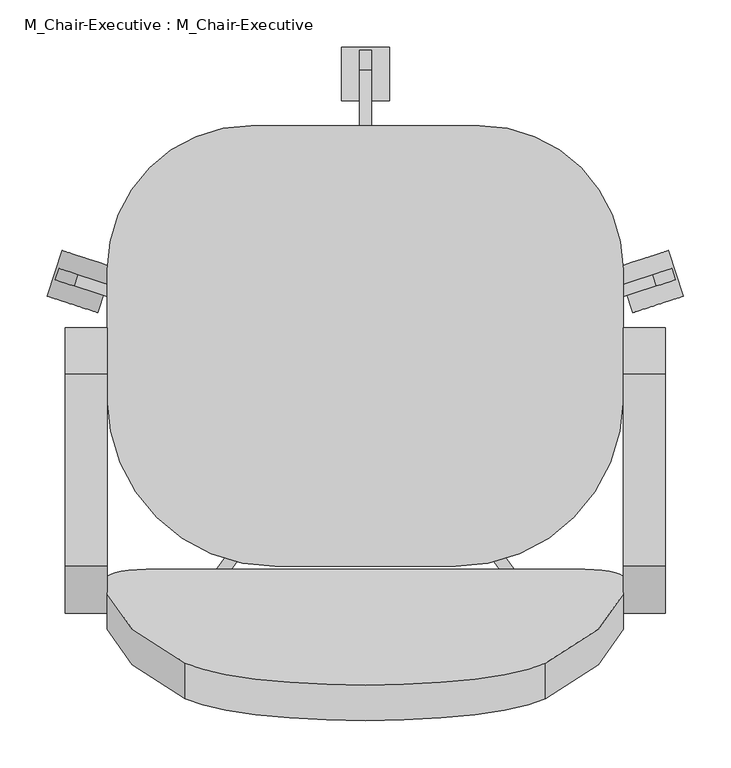
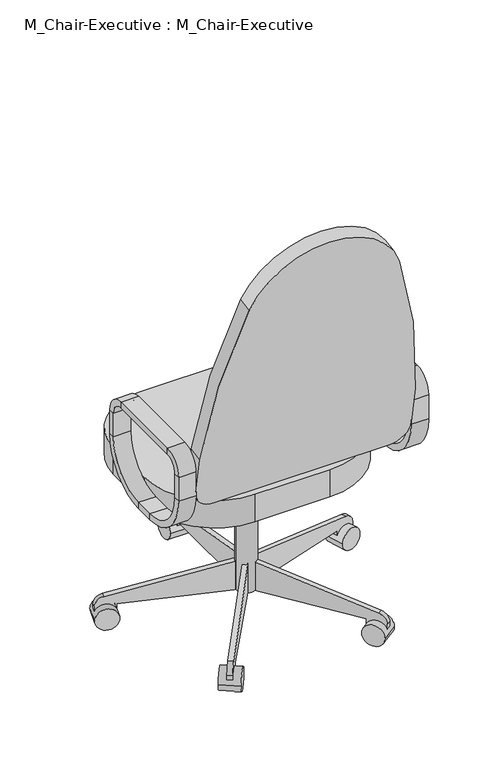
"""IFC4 building model written with IfcOpenShell, lengths in millimetres: furniture geometry, M_Chair-Executive : M_Chair-Executive."""

from ifc_helpers import new_model, si_unit, point, frame, frame_2d, origin, place, context, project, spatial, polyline, circle_curve, trimmed, segment, composite_curve, outline, extrude, source, transform, mapped, element, save
from ifc_brep_helpers import plane_surface, cylinder_surface, revolved_surface, advanced_brep


def m_chair_executive_m_chair_executive_8d69e98c(model_context):
    return source(origin(), model_context, "Body", "SolidModel", [
        advanced_brep(
        [(-176.5091803, -217.7873012, 546.1), (-176.5091803, -108.0540984, 436.3667972), (-176.5091803, -108.0540984, 420.4917972), (-176.5091803, -233.6623012, 546.1), (-132.0591803, -217.7873012, 546.1), (-132.0591803, -108.0540984, 436.3667972), (-132.0591803, -233.6623012, 546.1), (-132.0591803, -108.0540984, 420.4917972), (-176.5091803, -233.6623012, 609.6), (-176.5091803, -217.7873012, 609.6), (-132.0591803, -217.7873012, 609.6), (-132.0591803, -233.6623012, 609.6), (-176.5091803, -184.2540984, 643.1332028), (-176.5091803, -184.2540984, 659.0082028), (-132.0591803, -184.2540984, 643.1332028), (-132.0591803, -184.2540984, 659.0082028), (-176.5091803, 18.9459016, 659.0082028), (-176.5091803, 18.9459016, 643.1332028), (-132.0591803, 18.9459016, 643.1332028), (-132.0591803, 18.9459016, 659.0082028), (-176.5091803, 52.4791044, 609.6), (-176.5091803, 68.3541044, 609.6), (-132.0591803, 52.4791044, 609.6), (-132.0591803, 68.3541044, 609.6), (-176.5091803, 68.3541044, 546.1), (-176.5091803, 52.4791044, 546.1), (-132.0591803, 52.4791044, 546.1), (-132.0591803, 68.3541044, 546.1), (-176.5091803, -57.2540984, 436.3667972), (-176.5091803, -57.2540984, 420.4917972), (-132.0591803, -57.2540984, 436.3667972), (-132.0591803, -57.2540984, 420.4917972)],
        [
            (0, 1, circle_curve(frame((-176.5091803, -108.0540984, 546.1), z_axis=(1.0, 0.0, 0.0), x_axis=(0.0, 0.0, -1.0)), 109.7332028)),
            (1, 2),
            (2, 3, circle_curve(frame((-176.5091803, -108.0540984, 546.1), z_axis=(-1.0, 0.0, 0.0), x_axis=(0.0, 0.0, -1.0)), 125.6082028)),
            (3, 0),
            (4, 5, circle_curve(frame((-132.0591803, -108.0540984, 546.1), z_axis=(1.0, 0.0, 0.0), x_axis=(0.0, 0.0, -1.0)), 109.7332028)),
            (5, 1),
            (0, 4),
            (6, 7, circle_curve(frame((-132.0591803, -108.0540984, 546.1), z_axis=(1.0, 0.0, 0.0), x_axis=(0.0, 0.0, -1.0)), 125.6082028)),
            (7, 5),
            (4, 6),
            (2, 7),
            (6, 3),
            (3, 8),
            (8, 9),
            (9, 0),
            (9, 10),
            (10, 4),
            (10, 11),
            (11, 6),
            (11, 8),
            (12, 9, circle_curve(frame((-176.5091803, -184.2540984, 609.6), z_axis=(1.0, 0.0, 0.0), x_axis=(0.0, -1.0, 0.0)), 33.5332028)),
            (8, 13, circle_curve(frame((-176.5091803, -184.2540984, 609.6), z_axis=(-1.0, 0.0, 0.0), x_axis=(0.0, -1.0, 0.0)), 49.4082028)),
            (13, 12),
            (14, 10, circle_curve(frame((-132.0591803, -184.2540984, 609.6), z_axis=(1.0, 0.0, 0.0), x_axis=(0.0, -1.0, 0.0)), 33.5332028)),
            (12, 14),
            (15, 11, circle_curve(frame((-132.0591803, -184.2540984, 609.6), z_axis=(1.0, 0.0, 0.0), x_axis=(0.0, -1.0, 0.0)), 49.4082028)),
            (14, 15),
            (15, 13),
            (13, 16),
            (16, 17),
            (17, 12),
            (17, 18),
            (18, 14),
            (18, 19),
            (19, 15),
            (19, 16),
            (20, 17, circle_curve(frame((-176.5091803, 18.9459016, 609.6), z_axis=(1.0, 0.0, 0.0), x_axis=(0.0, 0.0, 1.0)), 33.5332028)),
            (16, 21, circle_curve(frame((-176.5091803, 18.9459016, 609.6), z_axis=(-1.0, 0.0, 0.0), x_axis=(0.0, 0.0, 1.0)), 49.4082028)),
            (21, 20),
            (22, 18, circle_curve(frame((-132.0591803, 18.9459016, 609.6), z_axis=(1.0, 0.0, 0.0), x_axis=(0.0, 0.0, 1.0)), 33.5332028)),
            (20, 22),
            (23, 19, circle_curve(frame((-132.0591803, 18.9459016, 609.6), z_axis=(1.0, 0.0, 0.0), x_axis=(0.0, 0.0, 1.0)), 49.4082028)),
            (22, 23),
            (23, 21),
            (21, 24),
            (24, 25),
            (25, 20),
            (25, 26),
            (26, 22),
            (26, 27),
            (27, 23),
            (27, 24),
            (28, 25, circle_curve(frame((-176.5091803, -57.2540984, 546.1), z_axis=(1.0, 0.0, 0.0), x_axis=(0.0, 1.0, 0.0)), 109.7332028)),
            (24, 29, circle_curve(frame((-176.5091803, -57.2540984, 546.1), z_axis=(-1.0, 0.0, 0.0), x_axis=(0.0, 1.0, 0.0)), 125.6082028)),
            (29, 28),
            (30, 26, circle_curve(frame((-132.0591803, -57.2540984, 546.1), z_axis=(1.0, 0.0, 0.0), x_axis=(0.0, 1.0, 0.0)), 109.7332028)),
            (28, 30),
            (31, 27, circle_curve(frame((-132.0591803, -57.2540984, 546.1), z_axis=(1.0, 0.0, 0.0), x_axis=(0.0, 1.0, 0.0)), 125.6082028)),
            (30, 31),
            (31, 29),
            (29, 2),
            (1, 28),
            (5, 30),
            (7, 31),
        ],
        [
            plane_surface(frame((-176.5091803, -108.0540984, 546.1), z_axis=(-1.0, 0.0, 0.0), x_axis=(0.0, 0.0, -1.0))),
            revolved_surface(polyline([(-176.5091803, -108.0540984, 436.3667972), (-132.0591803, -108.0540984, 436.3667972)]), (-132.0591803, -108.0540984, 546.1), (-1.0, 0.0, 0.0)),
            plane_surface(frame((-132.0591803, -108.0540984, 546.1), z_axis=(1.0, 0.0, 0.0), x_axis=(0.0, 0.0, -1.0))),
            cylinder_surface(frame((-132.0591803, -108.0540984, 546.1), z_axis=(-1.0, 0.0, 0.0), x_axis=(0.0, 0.0, -1.0)), 125.6082028),
            plane_surface(frame((-176.5091803, -233.6623012, 546.1), z_axis=(-1.0, 0.0, 0.0), x_axis=(0.0, 0.0, 1.0))),
            plane_surface(frame((-176.5091803, -217.7873012, 546.1), z_axis=(0.0, 1.0, 0.0), x_axis=(0.0, 0.0, 1.0))),
            plane_surface(frame((-132.0591803, -217.7873012, 546.1), z_axis=(1.0, 0.0, 0.0), x_axis=(0.0, 0.0, 1.0))),
            plane_surface(frame((-132.0591803, -233.6623012, 546.1), z_axis=(0.0, -1.0, 0.0), x_axis=(0.0, 0.0, 1.0))),
            plane_surface(frame((-176.5091803, -184.2540984, 609.6), z_axis=(-1.0, 0.0, 0.0), x_axis=(0.0, -1.0, 0.0))),
            revolved_surface(polyline([(-176.5091803, -217.7873012, 609.6), (-132.0591803, -217.7873012, 609.6)]), (-132.0591803, -184.2540984, 609.6), (-1.0, 0.0, 0.0)),
            plane_surface(frame((-132.0591803, -184.2540984, 609.6), z_axis=(1.0, 0.0, 0.0), x_axis=(0.0, -1.0, 0.0))),
            cylinder_surface(frame((-132.0591803, -184.2540984, 609.6), z_axis=(-1.0, 0.0, 0.0), x_axis=(0.0, -1.0, 0.0)), 49.4082028),
            plane_surface(frame((-176.5091803, -184.2540984, 659.0082028), z_axis=(-1.0, 0.0, 0.0), x_axis=(0.0, 1.0, 0.0))),
            plane_surface(frame((-176.5091803, -184.2540984, 643.1332028), z_axis=(0.0, 0.0, -1.0), x_axis=(0.0, 1.0, 0.0))),
            plane_surface(frame((-132.0591803, -184.2540984, 643.1332028), z_axis=(1.0, 0.0, 0.0), x_axis=(0.0, 1.0, 0.0))),
            plane_surface(frame((-132.0591803, -184.2540984, 659.0082028), z_axis=(0.0, 0.0, 1.0), x_axis=(0.0, 1.0, 0.0))),
            plane_surface(frame((-176.5091803, 18.9459016, 609.6), z_axis=(-1.0, 0.0, 0.0), x_axis=(0.0, 0.0, 1.0))),
            revolved_surface(polyline([(-176.5091803, 18.9459016, 643.1332028), (-132.0591803, 18.9459016, 643.1332028)]), (-132.0591803, 18.9459016, 609.6), (-1.0, 0.0, 0.0)),
            plane_surface(frame((-132.0591803, 18.9459016, 609.6), z_axis=(1.0, 0.0, 0.0), x_axis=(0.0, 0.0, 1.0))),
            cylinder_surface(frame((-132.0591803, 18.9459016, 609.6), z_axis=(-1.0, 0.0, 0.0), x_axis=(0.0, 0.0, 1.0)), 49.4082028),
            plane_surface(frame((-176.5091803, 68.3541044, 609.6), z_axis=(-1.0, 0.0, 0.0), x_axis=(0.0, 0.0, -1.0))),
            plane_surface(frame((-176.5091803, 52.4791044, 609.6), z_axis=(0.0, -1.0, 0.0), x_axis=(0.0, 0.0, -1.0))),
            plane_surface(frame((-132.0591803, 52.4791044, 609.6), z_axis=(1.0, 0.0, 0.0), x_axis=(0.0, 0.0, -1.0))),
            plane_surface(frame((-132.0591803, 68.3541044, 609.6), z_axis=(0.0, 1.0, 0.0), x_axis=(0.0, 0.0, -1.0))),
            plane_surface(frame((-176.5091803, -57.2540984, 546.1), z_axis=(-1.0, 0.0, 0.0), x_axis=(0.0, 1.0, 0.0))),
            revolved_surface(polyline([(-176.5091803, 52.479104400000004, 546.1), (-132.0591803, 52.479104400000004, 546.1)]), (-132.0591803, -57.2540984, 546.1), (-1.0, 0.0, 0.0)),
            plane_surface(frame((-132.0591803, -57.2540984, 546.1), z_axis=(1.0, 0.0, 0.0), x_axis=(0.0, 1.0, 0.0))),
            cylinder_surface(frame((-132.0591803, -57.2540984, 546.1), z_axis=(-1.0, 0.0, 0.0), x_axis=(0.0, 1.0, 0.0)), 125.6082028),
            plane_surface(frame((-176.5091803, -57.2540984, 420.4917972), z_axis=(-1.0, 0.0, 0.0), x_axis=(0.0, -1.0, 0.0))),
            plane_surface(frame((-176.5091803, -57.2540984, 436.3667972), z_axis=(0.0, 0.0, 1.0), x_axis=(0.0, -1.0, 0.0))),
            plane_surface(frame((-132.0591803, -57.2540984, 436.3667972), z_axis=(1.0, 0.0, 0.0), x_axis=(0.0, -1.0, 0.0))),
            plane_surface(frame((-132.0591803, -57.2540984, 420.4917972), z_axis=(0.0, 0.0, -1.0), x_axis=(0.0, -1.0, 0.0))),
        ],
        [
            (0, [[1, 2, 3, 4]]),
            (1, [[5, 6, -1, 7]]),
            (2, [[8, 9, -5, 10]]),
            (3, [[-3, 11, -8, 12]]),
            (4, [[-4, 13, 14, 15]]),
            (5, [[-7, -15, 16, 17]]),
            (6, [[-10, -17, 18, 19]]),
            (7, [[-12, -19, 20, -13]]),
            (8, [[21, -14, 22, 23]]),
            (9, [[24, -16, -21, 25]]),
            (10, [[26, -18, -24, 27]]),
            (11, [[-22, -20, -26, 28]]),
            (12, [[-23, 29, 30, 31]]),
            (13, [[-25, -31, 32, 33]]),
            (14, [[-27, -33, 34, 35]]),
            (15, [[-28, -35, 36, -29]]),
            (16, [[37, -30, 38, 39]]),
            (17, [[40, -32, -37, 41]]),
            (18, [[42, -34, -40, 43]]),
            (19, [[-38, -36, -42, 44]]),
            (20, [[-39, 45, 46, 47]]),
            (21, [[-41, -47, 48, 49]]),
            (22, [[-43, -49, 50, 51]]),
            (23, [[-44, -51, 52, -45]]),
            (24, [[53, -46, 54, 55]]),
            (25, [[56, -48, -53, 57]]),
            (26, [[58, -50, -56, 59]]),
            (27, [[-54, -52, -58, 60]]),
            (28, [[-55, 61, -2, 62]]),
            (29, [[-57, -62, -6, 63]]),
            (30, [[-59, -63, -9, 64]]),
            (31, [[-60, -64, -11, -61]]),
        ],
    ),
        advanced_brep(
        [(414.0408197, -233.6623012, 546.1), (414.0408197, -108.0540984, 420.4917972), (458.4908197, -108.0540984, 420.4917972), (458.4908197, -233.6623012, 546.1), (414.0408197, -217.7873012, 546.1), (414.0408197, -108.0540984, 436.3667972), (458.4908197, -217.7873012, 546.1), (458.4908197, -108.0540984, 436.3667972), (458.4908197, -233.6623012, 609.6), (414.0408197, -233.6623012, 609.6), (414.0408197, -217.7873012, 609.6), (458.4908197, -217.7873012, 609.6), (414.0408197, -184.2540984, 659.0082028), (458.4908197, -184.2540984, 659.0082028), (414.0408197, -184.2540984, 643.1332028), (458.4908197, -184.2540984, 643.1332028), (458.4908197, 18.9459016, 659.0082028), (414.0408197, 18.9459016, 659.0082028), (414.0408197, 18.9459016, 643.1332028), (458.4908197, 18.9459016, 643.1332028), (414.0408197, 68.3541044, 609.6), (458.4908197, 68.3541044, 609.6), (414.0408197, 52.4791044, 609.6), (458.4908197, 52.4791044, 609.6), (458.4908197, 68.3541044, 546.1), (414.0408197, 68.3541044, 546.1), (414.0408197, 52.4791044, 546.1), (458.4908197, 52.4791044, 546.1), (414.0408197, -57.2540984, 420.4917972), (458.4908197, -57.2540984, 420.4917972), (414.0408197, -57.2540984, 436.3667972), (458.4908197, -57.2540984, 436.3667972)],
        [
            (0, 1, circle_curve(frame((414.0408197, -108.0540984, 546.1), z_axis=(1.0, 0.0, 0.0), x_axis=(0.0, 0.0, -1.0)), 125.6082028)),
            (1, 2),
            (2, 3, circle_curve(frame((458.4908197, -108.0540984, 546.1), z_axis=(-1.0, 0.0, 0.0), x_axis=(0.0, 0.0, -1.0)), 125.6082028)),
            (3, 0),
            (4, 5, circle_curve(frame((414.0408197, -108.0540984, 546.1), z_axis=(1.0, 0.0, 0.0), x_axis=(0.0, 0.0, -1.0)), 109.7332028)),
            (5, 1),
            (0, 4),
            (6, 7, circle_curve(frame((458.4908197, -108.0540984, 546.1), z_axis=(1.0, 0.0, 0.0), x_axis=(0.0, 0.0, -1.0)), 109.7332028)),
            (7, 5),
            (4, 6),
            (2, 7),
            (6, 3),
            (3, 8),
            (8, 9),
            (9, 0),
            (9, 10),
            (10, 4),
            (10, 11),
            (11, 6),
            (11, 8),
            (12, 9, circle_curve(frame((414.0408197, -184.2540984, 609.6), z_axis=(1.0, 0.0, 0.0), x_axis=(0.0, -1.0, 0.0)), 49.4082028)),
            (8, 13, circle_curve(frame((458.4908197, -184.2540984, 609.6), z_axis=(-1.0, 0.0, 0.0), x_axis=(0.0, -1.0, 0.0)), 49.4082028)),
            (13, 12),
            (14, 10, circle_curve(frame((414.0408197, -184.2540984, 609.6), z_axis=(1.0, 0.0, 0.0), x_axis=(0.0, -1.0, 0.0)), 33.5332028)),
            (12, 14),
            (15, 11, circle_curve(frame((458.4908197, -184.2540984, 609.6), z_axis=(1.0, 0.0, 0.0), x_axis=(0.0, -1.0, 0.0)), 33.5332028)),
            (14, 15),
            (15, 13),
            (13, 16),
            (16, 17),
            (17, 12),
            (17, 18),
            (18, 14),
            (18, 19),
            (19, 15),
            (19, 16),
            (20, 17, circle_curve(frame((414.0408197, 18.9459016, 609.6), z_axis=(1.0, 0.0, 0.0), x_axis=(0.0, 0.0, 1.0)), 49.4082028)),
            (16, 21, circle_curve(frame((458.4908197, 18.9459016, 609.6), z_axis=(-1.0, 0.0, 0.0), x_axis=(0.0, 0.0, 1.0)), 49.4082028)),
            (21, 20),
            (22, 18, circle_curve(frame((414.0408197, 18.9459016, 609.6), z_axis=(1.0, 0.0, 0.0), x_axis=(0.0, 0.0, 1.0)), 33.5332028)),
            (20, 22),
            (23, 19, circle_curve(frame((458.4908197, 18.9459016, 609.6), z_axis=(1.0, 0.0, 0.0), x_axis=(0.0, 0.0, 1.0)), 33.5332028)),
            (22, 23),
            (23, 21),
            (21, 24),
            (24, 25),
            (25, 20),
            (25, 26),
            (26, 22),
            (26, 27),
            (27, 23),
            (27, 24),
            (28, 25, circle_curve(frame((414.0408197, -57.2540984, 546.1), z_axis=(1.0, 0.0, 0.0), x_axis=(0.0, 1.0, 0.0)), 125.6082028)),
            (24, 29, circle_curve(frame((458.4908197, -57.2540984, 546.1), z_axis=(-1.0, 0.0, 0.0), x_axis=(0.0, 1.0, 0.0)), 125.6082028)),
            (29, 28),
            (30, 26, circle_curve(frame((414.0408197, -57.2540984, 546.1), z_axis=(1.0, 0.0, 0.0), x_axis=(0.0, 1.0, 0.0)), 109.7332028)),
            (28, 30),
            (31, 27, circle_curve(frame((458.4908197, -57.2540984, 546.1), z_axis=(1.0, 0.0, 0.0), x_axis=(0.0, 1.0, 0.0)), 109.7332028)),
            (30, 31),
            (31, 29),
            (29, 2),
            (1, 28),
            (5, 30),
            (7, 31),
        ],
        [
            cylinder_surface(frame((414.0408197, -108.0540984, 546.1), z_axis=(-1.0, 0.0, 0.0), x_axis=(0.0, 0.0, -1.0)), 125.6082028),
            plane_surface(frame((414.0408197, -108.0540984, 546.1), z_axis=(-1.0, 0.0, 0.0), x_axis=(0.0, 0.0, -1.0))),
            revolved_surface(polyline([(414.0408197, -108.0540984, 436.3667972), (458.4908197, -108.0540984, 436.3667972)]), (414.0408197, -108.0540984, 546.1), (-1.0, 0.0, 0.0)),
            plane_surface(frame((458.4908197, -108.0540984, 546.1), z_axis=(1.0, 0.0, 0.0), x_axis=(0.0, 0.0, -1.0))),
            plane_surface(frame((458.4908197, -233.6623012, 546.1), z_axis=(0.0, -1.0, 0.0), x_axis=(0.0, 0.0, 1.0))),
            plane_surface(frame((414.0408197, -233.6623012, 546.1), z_axis=(-1.0, 0.0, 0.0), x_axis=(0.0, 0.0, 1.0))),
            plane_surface(frame((414.0408197, -217.7873012, 546.1), z_axis=(0.0, 1.0, 0.0), x_axis=(0.0, 0.0, 1.0))),
            plane_surface(frame((458.4908197, -217.7873012, 546.1), z_axis=(1.0, 0.0, 0.0), x_axis=(0.0, 0.0, 1.0))),
            cylinder_surface(frame((414.0408197, -184.2540984, 609.6), z_axis=(-1.0, 0.0, 0.0), x_axis=(0.0, -1.0, 0.0)), 49.4082028),
            plane_surface(frame((414.0408197, -184.2540984, 609.6), z_axis=(-1.0, 0.0, 0.0), x_axis=(0.0, -1.0, 0.0))),
            revolved_surface(polyline([(414.0408197, -217.7873012, 609.6), (458.4908197, -217.7873012, 609.6)]), (414.0408197, -184.2540984, 609.6), (-1.0, 0.0, 0.0)),
            plane_surface(frame((458.4908197, -184.2540984, 609.6), z_axis=(1.0, 0.0, 0.0), x_axis=(0.0, -1.0, 0.0))),
            plane_surface(frame((458.4908197, -184.2540984, 659.0082028), z_axis=(0.0, 0.0, 1.0), x_axis=(0.0, 1.0, 0.0))),
            plane_surface(frame((414.0408197, -184.2540984, 659.0082028), z_axis=(-1.0, 0.0, 0.0), x_axis=(0.0, 1.0, 0.0))),
            plane_surface(frame((414.0408197, -184.2540984, 643.1332028), z_axis=(0.0, 0.0, -1.0), x_axis=(0.0, 1.0, 0.0))),
            plane_surface(frame((458.4908197, -184.2540984, 643.1332028), z_axis=(1.0, 0.0, 0.0), x_axis=(0.0, 1.0, 0.0))),
            cylinder_surface(frame((414.0408197, 18.9459016, 609.6), z_axis=(-1.0, 0.0, 0.0), x_axis=(0.0, 0.0, 1.0)), 49.4082028),
            plane_surface(frame((414.0408197, 18.9459016, 609.6), z_axis=(-1.0, 0.0, 0.0), x_axis=(0.0, 0.0, 1.0))),
            revolved_surface(polyline([(414.0408197, 18.9459016, 643.1332028), (458.4908197, 18.9459016, 643.1332028)]), (414.0408197, 18.9459016, 609.6), (-1.0, 0.0, 0.0)),
            plane_surface(frame((458.4908197, 18.9459016, 609.6), z_axis=(1.0, 0.0, 0.0), x_axis=(0.0, 0.0, 1.0))),
            plane_surface(frame((458.4908197, 68.3541044, 609.6), z_axis=(0.0, 1.0, 0.0), x_axis=(0.0, 0.0, -1.0))),
            plane_surface(frame((414.0408197, 68.3541044, 609.6), z_axis=(-1.0, 0.0, 0.0), x_axis=(0.0, 0.0, -1.0))),
            plane_surface(frame((414.0408197, 52.4791044, 609.6), z_axis=(0.0, -1.0, 0.0), x_axis=(0.0, 0.0, -1.0))),
            plane_surface(frame((458.4908197, 52.4791044, 609.6), z_axis=(1.0, 0.0, 0.0), x_axis=(0.0, 0.0, -1.0))),
            cylinder_surface(frame((414.0408197, -57.2540984, 546.1), z_axis=(-1.0, 0.0, 0.0), x_axis=(0.0, 1.0, 0.0)), 125.6082028),
            plane_surface(frame((414.0408197, -57.2540984, 546.1), z_axis=(-1.0, 0.0, 0.0), x_axis=(0.0, 1.0, 0.0))),
            revolved_surface(polyline([(414.0408197, 52.479104400000004, 546.1), (458.4908197, 52.479104400000004, 546.1)]), (414.0408197, -57.2540984, 546.1), (-1.0, 0.0, 0.0)),
            plane_surface(frame((458.4908197, -57.2540984, 546.1), z_axis=(1.0, 0.0, 0.0), x_axis=(0.0, 1.0, 0.0))),
            plane_surface(frame((458.4908197, -57.2540984, 420.4917972), z_axis=(0.0, 0.0, -1.0), x_axis=(0.0, -1.0, 0.0))),
            plane_surface(frame((414.0408197, -57.2540984, 420.4917972), z_axis=(-1.0, 0.0, 0.0), x_axis=(0.0, -1.0, 0.0))),
            plane_surface(frame((414.0408197, -57.2540984, 436.3667972), z_axis=(0.0, 0.0, 1.0), x_axis=(0.0, -1.0, 0.0))),
            plane_surface(frame((458.4908197, -57.2540984, 436.3667972), z_axis=(1.0, 0.0, 0.0), x_axis=(0.0, -1.0, 0.0))),
        ],
        [
            (0, [[1, 2, 3, 4]]),
            (1, [[5, 6, -1, 7]]),
            (2, [[8, 9, -5, 10]]),
            (3, [[-3, 11, -8, 12]]),
            (4, [[-4, 13, 14, 15]]),
            (5, [[-7, -15, 16, 17]]),
            (6, [[-10, -17, 18, 19]]),
            (7, [[-12, -19, 20, -13]]),
            (8, [[21, -14, 22, 23]]),
            (9, [[24, -16, -21, 25]]),
            (10, [[26, -18, -24, 27]]),
            (11, [[-22, -20, -26, 28]]),
            (12, [[-23, 29, 30, 31]]),
            (13, [[-25, -31, 32, 33]]),
            (14, [[-27, -33, 34, 35]]),
            (15, [[-28, -35, 36, -29]]),
            (16, [[37, -30, 38, 39]]),
            (17, [[40, -32, -37, 41]]),
            (18, [[42, -34, -40, 43]]),
            (19, [[-38, -36, -42, 44]]),
            (20, [[-39, 45, 46, 47]]),
            (21, [[-41, -47, 48, 49]]),
            (22, [[-43, -49, 50, 51]]),
            (23, [[-44, -51, 52, -45]]),
            (24, [[53, -46, 54, 55]]),
            (25, [[56, -48, -53, 57]]),
            (26, [[58, -50, -56, 59]]),
            (27, [[-54, -52, -58, 60]]),
            (28, [[-55, 61, -2, 62]]),
            (29, [[-57, -62, -6, 63]]),
            (30, [[-59, -63, -9, 64]]),
            (31, [[-60, -64, -11, -61]]),
        ],
    ),
        extrude(outline(composite_curve([segment(trimmed(circle_curve(frame_2d((0.0, -50.8)), 50.8), [point((0.0, 0.0))], [point((50.8, -50.8))], False, "CARTESIAN"), True, "CONTINUOUS"), segment(polyline([(50.8, -50.8), (50.8, -152.4)]), True, "CONTINUOUS"), segment(trimmed(circle_curve(frame_2d((-1471.2021854, -74.3913617)), 1524.0), [point((50.8, -152.4))], [point((-31.75, -574.9444618))], False, "CARTESIAN"), True, "CONTINUOUS"), segment(trimmed(circle_curve(frame_2d((-222.25, -504.2338544)), 203.2), [point((-31.75, -574.9444618))], [point((-412.75, -574.9444618))], False, "CARTESIAN"), True, "CONTINUOUS"), segment(trimmed(circle_curve(frame_2d((1026.7021854, -74.3913617)), 1524.0), [point((-412.75, -574.9444618))], [point((-495.3, -152.4))], False, "CARTESIAN"), True, "CONTINUOUS"), segment(polyline([(-495.3, -152.4), (-495.3, -50.8)]), True, "CONTINUOUS"), segment(trimmed(circle_curve(frame_2d((-444.5, -50.8)), 50.8), [point((-495.3, -50.8))], [point((-444.5, 0.0))], False, "CARTESIAN"), True, "CONTINUOUS"), segment(polyline([(-444.5, 0.0), (0.0, 0.0)]), True, "CONTINUOUS")], self_intersect=False)), frame((363.2408197, -224.5698964, 503.1641822), z_axis=(0.0, 0.9848077530122084, 0.17364817766692853), x_axis=(1.0, 0.0, 0.0)), (0.0, 0.0, 1.0), 38.1),
        extrude(outline(composite_curve([segment(trimmed(circle_curve(frame_2d((20.3408197, 129.4961016)), 152.4), [point((-132.0591803, 129.4961016))], [point((20.3408197, 281.8961016))], False, "CARTESIAN"), True, "CONTINUOUS"), segment(polyline([(20.3408197, 281.8961016), (261.6408197, 281.8961016)]), True, "CONTINUOUS"), segment(trimmed(circle_curve(frame_2d((261.6408197, 129.4961016)), 152.4), [point((261.6408197, 281.8961016))], [point((414.0408197, 129.4961016))], False, "CARTESIAN"), True, "CONTINUOUS"), segment(polyline([(414.0408197, 129.4961016), (414.0408197, -6.4540984)]), True, "CONTINUOUS"), segment(trimmed(circle_curve(frame_2d((236.2408197, -6.4540984)), 177.8), [point((414.0408197, -6.4540984))], [point((236.2408197, -184.2540984))], False, "CARTESIAN"), True, "CONTINUOUS"), segment(polyline([(236.2408197, -184.2540984), (45.7408197, -184.2540984)]), True, "CONTINUOUS"), segment(trimmed(circle_curve(frame_2d((45.7408197, -6.4540984)), 177.8), [point((45.7408197, -184.2540984))], [point((-132.0591803, -6.4540984))], False, "CARTESIAN"), True, "CONTINUOUS"), segment(polyline([(-132.0591803, -6.4540984), (-132.0591803, 129.4961016)]), True, "CONTINUOUS")], self_intersect=False)), frame((0.0, 0.0, 383.7835944), z_axis=(0.0, 0.0, 1.0), x_axis=(1.0, 0.0, 0.0)), (0.0, 0.0, 1.0), 73.4164056),
        extrude(outline(composite_curve([segment(trimmed(circle_curve(frame_2d((140.9908197, 18.9459016)), 25.4), [point((115.5908197, 18.9459016))], [point((166.3908197, 18.9459016))], False, "CARTESIAN"), True, "CONTINUOUS"), segment(trimmed(circle_curve(frame_2d((140.9908197, 18.9459016)), 25.4), [point((166.3908197, 18.9459016))], [point((115.5908197, 18.9459016))], False, "CARTESIAN"), True, "CONTINUOUS")], self_intersect=False)), frame((0.0, 0.0, 53.5835944), z_axis=(0.0, 0.0, 1.0), x_axis=(1.0, 0.0, 0.0)), (0.0, 0.0, 1.0), 330.5914056),
        extrude(outline(composite_curve([segment(trimmed(circle_curve(frame_2d((0.0, -28.2002727)), 28.2002727), [point((0.0, -56.4005455))], [point((0.0, 0.0))], False, "CARTESIAN"), True, "CONTINUOUS"), segment(trimmed(circle_curve(frame_2d((0.0, -28.2002727)), 28.2002727), [point((0.0, 0.0))], [point((0.0, -56.4005455))], False, "CARTESIAN"), True, "CONTINUOUS")], self_intersect=False)), frame((477.6203484, 101.6163254, 28.1835944), z_axis=(-0.3090169943749423, 0.9510565162951553, 0.0), x_axis=(0.0, 0.0, 1.0)), (0.0, 0.0, 1.0), 50.8),
        extrude(outline(composite_curve([segment(polyline([(-25.4, 0.0), (0.0, 0.0), (0.0, -50.8), (-24.303053, -50.8)]), True, "CONTINUOUS"), segment(trimmed(circle_curve(frame_2d((-24.303053, -25.4)), 25.4), [point((-24.303053, -50.8))], [point((-49.3171699, -29.8106637))], False, "CARTESIAN"), True, "CONTINUOUS"), segment(polyline([(-49.3171699, -29.8106637), (-101.6, 266.7), (-101.6, 292.1), (-25.4, 292.1), (-25.4, 0.0)]), True, "CONTINUOUS")], self_intersect=False)), frame((420.756686, 103.1705568, 28.1835944), z_axis=(-0.3090169943749423, 0.9510565162951553, 0.0), x_axis=(0.0, 0.0, -1.0)), (0.0, 0.0, 1.0), 12.7),
        extrude(outline(composite_curve([segment(trimmed(circle_curve(frame_2d((0.0, -28.2002727)), 28.2002727), [point((0.0, -56.4005455))], [point((0.0, 0.0))], False, "CARTESIAN"), True, "CONTINUOUS"), segment(trimmed(circle_curve(frame_2d((0.0, -28.2002727)), 28.2002727), [point((0.0, 0.0))], [point((0.0, -56.4005455))], False, "CARTESIAN"), True, "CONTINUOUS")], self_intersect=False)), frame((323.63931, -275.6612394, 28.1835944), z_axis=(0.8090169943749499, 0.5877852522924699, 0.0), x_axis=(0.0, 0.0, 1.0)), (0.0, 0.0, 1.0), 50.8),
        extrude(outline(composite_curve([segment(polyline([(-25.4, 0.0), (0.0, 0.0), (0.0, -50.8), (-24.303053, -50.8)]), True, "CONTINUOUS"), segment(trimmed(circle_curve(frame_2d((-24.303053, -25.3999999)), 25.4), [point((-24.303053, -50.8))], [point((-49.3171699, -29.8106636))], False, "CARTESIAN"), True, "CONTINUOUS"), segment(polyline([(-49.3171699, -29.8106636), (-101.6, 266.7), (-101.6, 292.1), (-25.4, 292.1), (-25.4, 0.0)]), True, "CONTINUOUS")], self_intersect=False)), frame((307.545634, -221.1003988, 28.1835944), z_axis=(0.8090169943749499, 0.5877852522924699, 0.0), x_axis=(0.0, 0.0, -1.0)), (0.0, 0.0, 1.0), 12.7),
        extrude(outline(composite_curve([segment(trimmed(circle_curve(frame_2d((0.0, -28.2002727)), 28.2002727), [point((0.0, -56.4005455))], [point((0.0, 0.0))], False, "CARTESIAN"), True, "CONTINUOUS"), segment(trimmed(circle_curve(frame_2d((0.0, -28.2002727)), 28.2002727), [point((0.0, 0.0))], [point((0.0, -56.4005455))], False, "CARTESIAN"), True, "CONTINUOUS")], self_intersect=False)), frame((-41.6576707, -275.6612394, 28.1835944), z_axis=(-0.8090169943749458, 0.5877852522924754, 0.0), x_axis=(0.0, 0.0, -1.0)), (0.0, 0.0, 1.0), 50.8),
        extrude(outline(composite_curve([segment(polyline([(25.4, 0.0), (25.4, 292.1), (101.6, 292.1), (101.6, 266.7), (49.3171699, -29.8106637)]), True, "CONTINUOUS"), segment(trimmed(circle_curve(frame_2d((24.303053, -25.3999999)), 25.4), [point((49.3171699, -29.8106637))], [point((24.303053, -50.8))], False, "CARTESIAN"), True, "CONTINUOUS"), segment(polyline([(24.303053, -50.8), (0.0, -50.8), (0.0, 0.0), (25.4, 0.0)]), True, "CONTINUOUS")], self_intersect=False)), frame((-25.5639946, -221.1003988, 28.1835944), z_axis=(-0.8090169943749459, 0.5877852522924754, 0.0), x_axis=(0.0, 0.0, 1.0)), (0.0, 0.0, 1.0), 12.7),
        extrude(outline(composite_curve([segment(trimmed(circle_curve(frame_2d((0.0, -28.2002727)), 28.2002727), [point((0.0, -56.4005454))], [point((0.0, 0.0))], False, "CARTESIAN"), True, "CONTINUOUS"), segment(trimmed(circle_curve(frame_2d((0.0, -28.2002727)), 28.2002727), [point((0.0, 0.0))], [point((0.0, -56.4005454))], False, "CARTESIAN"), True, "CONTINUOUS")], self_intersect=False)), frame((-195.638709, 101.6163254, 28.1835944), z_axis=(0.3090169943749487, 0.9510565162951532, 0.0), x_axis=(0.0, 0.0, -1.0)), (0.0, 0.0, 1.0), 50.8),
        extrude(outline(composite_curve([segment(polyline([(25.4, 0.0), (25.4, 292.1000001), (101.6, 292.1000001), (101.6, 266.7), (49.3171699, -29.8106636)]), True, "CONTINUOUS"), segment(trimmed(circle_curve(frame_2d((24.303053, -25.4)), 25.4), [point((49.3171699, -29.8106636))], [point((24.303053, -50.8))], False, "CARTESIAN"), True, "CONTINUOUS"), segment(polyline([(24.303053, -50.8), (0.0, -50.8), (0.0, 0.0), (25.4, 0.0)]), True, "CONTINUOUS")], self_intersect=False)), frame((-138.7750467, 103.1705568, 28.1835944), z_axis=(0.3090169943749487, 0.9510565162951532, 0.0), x_axis=(0.0, 0.0, 1.0)), (0.0, 0.0, 1.0), 12.7),
        extrude(outline(composite_curve([segment(trimmed(circle_curve(frame_2d((336.4459016, 28.1835944)), 28.2002727), [point((308.2456289, 28.1835944))], [point((364.6461744, 28.1835944))], False, "CARTESIAN"), True, "CONTINUOUS"), segment(trimmed(circle_curve(frame_2d((336.4459016, 28.1835944)), 28.2002727), [point((364.6461744, 28.1835944))], [point((308.2456289, 28.1835944))], False, "CARTESIAN"), True, "CONTINUOUS")], self_intersect=False)), frame((115.5908197, 0.0, 0.0), z_axis=(1.0, 0.0, 0.0), x_axis=(0.0, 1.0, 0.0)), (0.0, 0.0, 1.0), 50.8),
        extrude(outline(composite_curve([segment(polyline([(311.0459016, 53.5835944), (18.9459016, 53.5835944), (18.9459016, 129.7835944), (44.3459016, 129.7835944), (340.8565654, 77.5007643)]), True, "CONTINUOUS"), segment(trimmed(circle_curve(frame_2d((336.4459016, 52.4866474)), 25.4), [point((340.8565654, 77.5007643))], [point((361.8459016, 52.4866474))], False, "CARTESIAN"), True, "CONTINUOUS"), segment(polyline([(361.8459016, 52.4866474), (361.8459016, 28.1835944), (311.0459016, 28.1835944), (311.0459016, 53.5835944)]), True, "CONTINUOUS")], self_intersect=False)), frame((134.6408197, 0.0, 0.0), z_axis=(1.0, 0.0, 0.0), x_axis=(0.0, 1.0, 0.0)), (0.0, 0.0, 1.0), 12.7),
        extrude(outline(polyline([(69.7459016, 383.7835944), (69.7459016, 371.0835944), (18.9459016, 283.0954134), (-19.1540984, 283.0954134), (-19.1540984, 383.7835944), (69.7459016, 383.7835944)])), frame((90.1908197, 0.0, 0.0), z_axis=(1.0, 0.0, 0.0), x_axis=(0.0, 1.0, 0.0)), (0.0, 0.0, 1.0), 101.6),
    ])


if __name__ == "__main__":
    model = new_model("IFC4")
    model_context = context("Model", 3, world=origin())
    ifc_project = project(units=[si_unit("LENGTHUNIT", "METRE", prefix="MILLI")], contexts=[model_context])
    site = spatial("IfcSite", under=ifc_project)
    building = spatial("IfcBuilding", under=site)
    placement = place(None, origin())
    m_chair_executive_m_chair_executive_shape = m_chair_executive_m_chair_executive_8d69e98c(model_context)
    element("IfcFurniture", 1, ObjectType="M_Chair-Executive : M_Chair-Executive", at=placement, inside=building, context=model_context, shape_type="MappedRepresentation", body=[
        mapped(m_chair_executive_m_chair_executive_shape, transform((0.0, 0.0, 0.0), x_axis=(1.0, 0.0, 0.0), y_axis=(0.0, 1.0, 0.0), z_axis=(0.0, 0.0, 1.0))),
    ])
    save(model, "model.ifc")

# Revit data of these elements
# Type "M_Chair-Executive : M_Chair-Executive"
#   Base/Armd Material = Plastic, Opaque Black
#   Caster Material = Plastic, Opaque Black
#   Seat/Back Material = Textile - Slate Blue
#   Default Elevation = 0
# Element 1 (IfcFurniture, "M_Chair-Executive : M_Chair-Executive")
#   Materials on its faces: "Plastic, Opaque Black", "Textile - Slate Blue"
# Materials
#   "Plastic, Opaque Black": class "Plastic", colour RGB 0 0 0, transparency 0.7, Description = "Plastic, generic, opaque black", Cost = 0
#   "Textile - Slate Blue": class "Fabric", colour RGB 98 102 118, transparency 0
